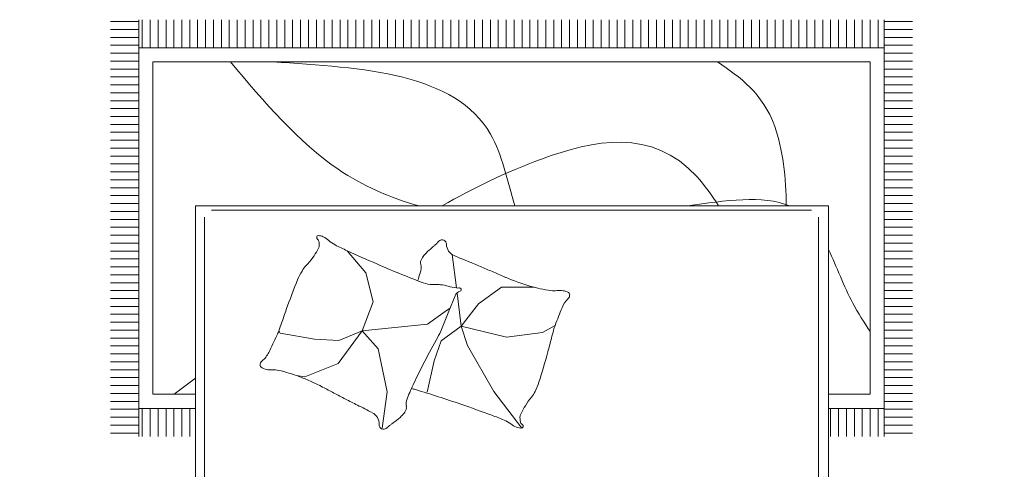
# Model space of a CAD drawing. Units: inches. Extents: x -7 to 1228, y -146 to 1091.
# Tile 78 of 88: x 656 to 743, y 890 to 929. Entities that reach past the tile are written whole.
import ezdxf

# ---------------------------------------------------------------- set-up
doc = ezdxf.new("R2010")
doc.units = ezdxf.units.IN
doc.layers.add('A-FURN', color=8, linetype='Continuous', lineweight=18)
doc.styles.add('DIM_FONT', font='SIMPLEX.shx', dxfattribs={"width": 0.8})

# ---------------------------------------------------------------- blocks, each defined once
blk = doc.blocks.new('A$C4F634EDD')
for p, q in [((0, 2.6295), (0, 2.2295)), ((0.5, 2.6295), (0, 2.6295)), ((0.5, 2.6295), (2.3, 2.6295)), ((0.5, 0.5295), (0.5, 2.6295)), ((0.5, 2.2295), (0.5, 2.6295)), ((2.3, 2.6295), (2.3, 0.5295)), ((2.3, 2.6295), (2.8, 2.6295)), ((2.3, 2.2295), (2.3, 2.6295)), ((2.8, 2.6295), (2.8, 2.2295)), ((0.5, 2.5771), (2.3, 2.5771)), ((2.392, 2.5115), (2.5692, 2.5765)), ((2.5692, 2.5765), (2.574, 2.5743)), ((0.2457, 2.5697), (0.2457, 2.4733)), ((2.4985, 2.5445), (2.5516, 2.564)), ((2.5062, 2.5454), (2.5487, 2.561)), ((2.5483, 2.5347), (2.5487, 2.561)), ((2.5487, 2.561), (2.5571, 2.56)), ((2.5615, 2.5536), (2.5514, 2.5318)), ((2.5516, 2.564), (2.5637, 2.5584)), ((2.5571, 2.56), (2.5615, 2.5536)), ((2.5615, 2.5536), (2.5791, 2.5058)), ((2.5637, 2.5584), (2.6418, 2.3458)), ((2.574, 2.5743), (2.6638, 2.3298)), ((2.4842, 2.5232), (2.47, 2.518)), ((2.4862, 2.5179), (2.4842, 2.5232)), ((2.4946, 2.5331), (2.4985, 2.5445)), ((2.5734, 2.3187), (2.4946, 2.5331)), ((2.5062, 2.5454), (2.5004, 2.5392)), ((2.5004, 2.5392), (2.5013, 2.5315)), ((2.5013, 2.5315), (2.5188, 2.4836)), ((2.5013, 2.5315), (2.5231, 2.5214)), ((2.5235, 2.5256), (2.5062, 2.5454)), ((2.5231, 2.5214), (2.5235, 2.5256)), ((2.5523, 2.4417), (2.5231, 2.5214)), ((2.5483, 2.5347), (2.5235, 2.5256)), ((2.5514, 2.5318), (2.5483, 2.5347)), ((2.5807, 2.4521), (2.5514, 2.5318)), ((2.3898, 2.5066), (2.392, 2.5115)), ((2.4795, 2.2621), (2.3898, 2.5066)), ((2.412, 2.5007), (2.4634, 2.5196)), ((2.4361, 2.4352), (2.412, 2.5007)), ((2.4634, 2.5196), (2.4875, 2.454)), ((2.47, 2.518), (2.472, 2.5127)), ((2.472, 2.5127), (2.4862, 2.5179)), ((2.4881, 2.5126), (2.4739, 2.5074)), ((2.4739, 2.5074), (2.4759, 2.502)), ((2.4759, 2.502), (2.4901, 2.5073)), ((2.492, 2.5019), (2.4778, 2.4967)), ((2.4778, 2.4967), (2.4798, 2.4914)), ((2.4798, 2.4914), (2.494, 2.4966)), ((2.4901, 2.5073), (2.4881, 2.5126)), ((2.494, 2.4966), (2.492, 2.5019)), ((2.5788, 2.4956), (2.5767, 2.4848)), ((2.5791, 2.5058), (2.5788, 2.4956)), ((2.4959, 2.4913), (2.4817, 2.4861)), ((2.4817, 2.4861), (2.4837, 2.4808)), ((2.4837, 2.4808), (2.4979, 2.486)), ((2.4998, 2.4807), (2.4856, 2.4755)), ((2.4856, 2.4755), (2.4876, 2.4702)), ((2.4876, 2.4702), (2.5018, 2.4754)), ((2.5037, 2.47), (2.4895, 2.4648)), ((2.4895, 2.4648), (2.4915, 2.4595)), ((2.4915, 2.4595), (2.5057, 2.4647)), ((2.4979, 2.486), (2.4959, 2.4913)), ((2.5018, 2.4754), (2.4998, 2.4807)), ((2.5057, 2.4647), (2.5037, 2.47)), ((2.5188, 2.4836), (2.5256, 2.4761)), ((2.5256, 2.4761), (2.5342, 2.4692)), ((2.5342, 2.4692), (2.5405, 2.4574)), ((2.5767, 2.4848), (2.5795, 2.4717)), ((2.5795, 2.4717), (2.586, 2.454)), ((2.4875, 2.454), (2.4361, 2.4352)), ((2.5405, 2.4574), (2.547, 2.4397)), ((2.5594, 2.4061), (2.547, 2.4397)), ((2.5523, 2.4417), (2.5875, 2.346)), ((2.5807, 2.4521), (2.6158, 2.3564)), ((2.5984, 2.4204), (2.586, 2.454)), ((0.0957, 2.4197), (0.192, 2.4197)), ((0.2994, 2.4197), (0.3957, 2.4197)), ((2.4457, 2.4146), (2.4563, 2.4185)), ((2.4496, 2.4039), (2.4457, 2.4146)), ((2.4563, 2.4185), (2.4602, 2.4078)), ((2.4634, 2.4211), (2.474, 2.425)), ((2.4673, 2.4104), (2.4634, 2.4211)), ((2.4779, 2.4143), (2.4673, 2.4104)), ((2.474, 2.425), (2.4779, 2.4143)), ((2.4811, 2.4276), (2.4917, 2.4315)), ((2.485, 2.4169), (2.4811, 2.4276)), ((2.4956, 2.4208), (2.485, 2.4169)), ((2.4883, 2.4081), (2.4989, 2.412)), ((2.4922, 2.3975), (2.4883, 2.4081)), ((2.4917, 2.4315), (2.4956, 2.4208)), ((2.4989, 2.412), (2.5028, 2.4014)), ((2.6047, 2.4086), (2.5984, 2.4204)), ((2.6133, 2.4017), (2.6047, 2.4086)), ((2.4602, 2.4078), (2.4496, 2.4039)), ((2.4528, 2.3951), (2.4635, 2.399)), ((2.4567, 2.3844), (2.4528, 2.3951)), ((2.4674, 2.3883), (2.4567, 2.3844)), ((2.4635, 2.399), (2.4674, 2.3883)), ((2.4706, 2.4016), (2.4812, 2.4055)), ((2.4745, 2.3909), (2.4706, 2.4016)), ((2.4851, 2.3949), (2.4745, 2.3909)), ((2.4777, 2.3821), (2.4883, 2.386)), ((2.4816, 2.3715), (2.4777, 2.3821)), ((2.4812, 2.4055), (2.4851, 2.3949)), ((2.4883, 2.386), (2.4922, 2.3754)), ((2.5028, 2.4014), (2.4922, 2.3975)), ((2.4954, 2.3886), (2.5061, 2.3925)), ((2.4993, 2.378), (2.4954, 2.3886)), ((2.51, 2.3819), (2.4993, 2.378)), ((2.5061, 2.3925), (2.51, 2.3819)), ((2.5238, 2.3769), (2.538, 2.3821)), ((2.538, 2.3821), (2.5419, 2.3715)), ((2.5622, 2.393), (2.5594, 2.4061)), ((2.5598, 2.372), (2.5601, 2.3822)), ((2.5601, 2.3822), (2.5622, 2.393)), ((2.6201, 2.3941), (2.6133, 2.4017)), ((2.6376, 2.3463), (2.6201, 2.3941)), ((2.6499, 2.3979), (2.6397, 2.3953)), ((2.6417, 2.39), (2.6488, 2.391)), ((2.6488, 2.391), (2.6538, 2.3895)), ((2.6551, 2.397), (2.6499, 2.3979)), ((2.6538, 2.3895), (2.6596, 2.388)), ((2.6627, 2.392), (2.6551, 2.397)), ((2.6596, 2.388), (2.6626, 2.3867)), ((2.6626, 2.3867), (2.6662, 2.388)), ((2.6692, 2.394), (2.6627, 2.392)), ((2.6662, 2.388), (2.6632, 2.3828)), ((2.6632, 2.3828), (2.6736, 2.3744)), ((2.6736, 2.3944), (2.6692, 2.394)), ((2.6765, 2.391), (2.6736, 2.3944)), ((2.6742, 2.3795), (2.6765, 2.391)), ((2.6824, 2.3858), (2.6742, 2.3795)), ((2.6873, 2.3815), (2.6824, 2.3858)), ((2.6853, 2.369), (2.6873, 2.3815)), ((0.2457, 2.366), (0.2457, 2.2697)), ((2.46, 2.3756), (2.4706, 2.3795)), ((2.4639, 2.365), (2.46, 2.3756)), ((2.4745, 2.3689), (2.4639, 2.365)), ((2.4672, 2.3561), (2.4778, 2.36)), ((2.4711, 2.3455), (2.4672, 2.3561)), ((2.4706, 2.3795), (2.4745, 2.3689)), ((2.4778, 2.36), (2.4817, 2.3494)), ((2.4922, 2.3754), (2.4816, 2.3715)), ((2.4849, 2.3626), (2.4955, 2.3665)), ((2.4888, 2.352), (2.4849, 2.3626)), ((2.4994, 2.3559), (2.4888, 2.352)), ((2.4955, 2.3665), (2.4994, 2.3559)), ((2.5026, 2.3691), (2.5132, 2.373)), ((2.5065, 2.3585), (2.5026, 2.3691)), ((2.5171, 2.3624), (2.5065, 2.3585)), ((2.5132, 2.373), (2.5171, 2.3624)), ((2.5277, 2.3663), (2.5238, 2.3769)), ((2.5419, 2.3715), (2.5277, 2.3663)), ((2.5774, 2.3242), (2.5598, 2.372)), ((2.6154, 2.3522), (2.5905, 2.3431)), ((2.6158, 2.3564), (2.6154, 2.3522)), ((2.6154, 2.3522), (2.6327, 2.3324)), ((2.6376, 2.3463), (2.6158, 2.3564)), ((2.6736, 2.3744), (2.6922, 2.3593)), ((2.6946, 2.376), (2.6853, 2.369)), ((2.6922, 2.3593), (2.7051, 2.3473)), ((2.6995, 2.3713), (2.6946, 2.376)), ((2.695, 2.3603), (2.6995, 2.3713)), ((2.7031, 2.3682), (2.695, 2.3603)), ((2.7096, 2.3616), (2.7031, 2.3682)), ((2.7062, 2.351), (2.7096, 2.3616)), ((2.7147, 2.3578), (2.7062, 2.351)), ((2.7214, 2.3517), (2.7147, 2.3578)), ((0, 2.3301), (0.5, 2.3301)), ((2.8, 2.3301), (2.3, 2.3301)), ((2.4817, 2.3494), (2.4711, 2.3455)), ((2.5774, 2.3242), (2.5875, 2.346)), ((2.5818, 2.3178), (2.5774, 2.3242)), ((2.5875, 2.346), (2.5905, 2.3431)), ((2.5905, 2.3431), (2.5901, 2.3168)), ((2.5901, 2.3168), (2.6097, 2.324)), ((2.613, 2.3312), (2.6077, 2.3293)), ((2.6077, 2.3293), (2.6135, 2.3141)), ((2.6192, 2.3174), (2.613, 2.3312)), ((2.6153, 2.3261), (2.6327, 2.3324)), ((2.6369, 2.332), (2.6161, 2.3243)), ((2.6616, 2.3249), (2.6234, 2.3109)), ((2.6327, 2.3324), (2.6385, 2.3386)), ((2.6418, 2.3458), (2.6369, 2.332)), ((2.6385, 2.3386), (2.6376, 2.3463)), ((2.6638, 2.3298), (2.6616, 2.3249)), ((2.7051, 2.3473), (2.7079, 2.3475)), ((2.7079, 2.3475), (2.7079, 2.3443)), ((2.7079, 2.3443), (2.727, 2.3277)), ((2.7196, 2.34), (2.7214, 2.3517)), ((2.7286, 2.3466), (2.7196, 2.34)), ((2.727, 2.3277), (2.7512, 2.2983)), ((2.7346, 2.3423), (2.7286, 2.3466)), ((2.732, 2.3295), (2.7346, 2.3423)), ((2.7423, 2.3345), (2.732, 2.3295)), ((2.7406, 2.3172), (2.7495, 2.325)), ((2.7495, 2.325), (2.7423, 2.3345)), ((2.6172, 2.3086), (2.4844, 2.2599)), ((2.5362, 2.305), (2.5185, 2.2985)), ((2.5185, 2.2985), (2.5224, 2.2879)), ((2.5401, 2.2944), (2.5362, 2.305)), ((2.561, 2.3141), (2.5433, 2.3076)), ((2.5433, 2.3076), (2.5472, 2.297)), ((2.5472, 2.297), (2.5649, 2.3035)), ((2.5649, 2.3035), (2.561, 2.3141)), ((2.5855, 2.3131), (2.5734, 2.3187)), ((2.5901, 2.3168), (2.5818, 2.3178)), ((2.6104, 2.3222), (2.5855, 2.3131)), ((2.6135, 2.3141), (2.6244, 2.2977)), ((2.626, 2.3069), (2.6192, 2.3174)), ((2.6244, 2.2977), (2.6349, 2.2825)), ((2.6365, 2.2916), (2.626, 2.3069)), ((2.7519, 2.3218), (2.7406, 2.3172)), ((2.7512, 2.2983), (2.756, 2.2695)), ((2.7575, 2.3144), (2.7519, 2.3218)), ((2.7526, 2.3045), (2.7575, 2.3144)), ((2.7622, 2.308), (2.7526, 2.3045)), ((2.7574, 2.2924), (2.7673, 2.2997)), ((2.7673, 2.2997), (2.7622, 2.308)), ((0.5953, 2.1912), (0.616, 2.2738)), ((1.4546, 2.1912), (1.4752, 2.2738)), ((2.5114, 2.2959), (2.4936, 2.2894)), ((2.4936, 2.2894), (2.4976, 2.2788)), ((2.4976, 2.2788), (2.5153, 2.2853)), ((2.5153, 2.2853), (2.5114, 2.2959)), ((2.5224, 2.2879), (2.5401, 2.2944)), ((2.6349, 2.2825), (2.638, 2.273)), ((2.6407, 2.2834), (2.6365, 2.2916)), ((2.6399, 2.2712), (2.6374, 2.2659)), ((2.638, 2.273), (2.6399, 2.2712)), ((2.6438, 2.2739), (2.6407, 2.2834)), ((2.6519, 2.2716), (2.6438, 2.2739)), ((2.6535, 2.2628), (2.6519, 2.2716)), ((2.756, 2.2695), (2.7459, 2.2483)), ((2.7687, 2.2905), (2.7574, 2.2924)), ((2.7587, 2.279), (2.7699, 2.2828)), ((2.7708, 2.2725), (2.7587, 2.279)), ((2.7699, 2.2828), (2.7687, 2.2905)), ((2.7706, 2.2643), (2.7708, 2.2725)), ((2.4844, 2.2599), (2.4795, 2.2621)), ((2.6374, 2.2659), (2.6398, 2.257)), ((2.6398, 2.257), (2.6509, 2.259)), ((2.6509, 2.259), (2.6431, 2.2492)), ((2.6431, 2.2492), (2.6473, 2.2398)), ((2.6473, 2.2398), (2.6592, 2.2429)), ((2.6592, 2.2429), (2.6521, 2.2314)), ((2.6636, 2.2409), (2.6535, 2.2628)), ((2.6836, 2.2287), (2.6636, 2.2409)), ((2.7459, 2.2483), (2.7284, 2.2317)), ((2.7509, 2.2314), (2.7459, 2.2418)), ((2.7459, 2.2418), (2.7568, 2.2352)), ((2.7529, 2.2505), (2.7645, 2.2498)), ((2.7607, 2.2424), (2.7529, 2.2505)), ((2.7568, 2.2352), (2.7607, 2.2424)), ((2.759, 2.2637), (2.7706, 2.2643)), ((2.7676, 2.2559), (2.759, 2.2637)), ((2.7645, 2.2498), (2.7676, 2.2559)), ((0, 2.2295), (0.5, 2.2295)), ((2.8, 2.2295), (2.3, 2.2295)), ((2.6521, 2.2314), (2.6598, 2.2248)), ((2.6598, 2.2248), (2.6697, 2.2309)), ((2.6697, 2.2309), (2.6684, 2.219)), ((2.6684, 2.219), (2.6761, 2.2145)), ((2.6761, 2.2145), (2.6821, 2.2237)), ((2.6821, 2.2237), (2.6843, 2.2135)), ((2.7063, 2.2256), (2.6836, 2.2287)), ((2.6843, 2.2135), (2.6927, 2.2117)), ((2.6927, 2.2117), (2.6986, 2.222)), ((2.6986, 2.222), (2.7019, 2.2098)), ((2.7284, 2.2317), (2.7063, 2.2256)), ((2.7102, 2.2104), (2.7113, 2.2218)), ((2.7113, 2.2218), (2.7192, 2.2137)), ((2.7192, 2.2137), (2.7255, 2.2152)), ((2.7255, 2.2152), (2.7242, 2.2265)), ((2.7242, 2.2265), (2.7324, 2.2165)), ((2.7324, 2.2165), (2.7386, 2.2208)), ((2.7386, 2.2208), (2.7354, 2.2306)), ((2.7354, 2.2306), (2.7462, 2.2264)), ((2.7462, 2.2264), (2.7509, 2.2314)), ((0.5878, 2.1612), (0.5953, 2.1912)), ((1.4471, 2.1612), (1.4546, 2.1912)), ((2.7019, 2.2098), (2.7102, 2.2104)), ((1.5035, 2.141), (0.5458, 2.141)), ((1.5035, 2.141), (2.2716, 1.7136)), ((0.5258, 2.121), (0.5258, 0.5617)), ((1.576, 1.9433), (1.5624, 1.8479)), ((0.5458, 1.8684), (1.5653, 1.8684)), ((1.5624, 1.8479), (1.5641, 1.7178)), ((2.2716, 0.5617), (2.2716, 1.7136)), ((0.3386, 0), (0.3386, 1.1852)), ((0.3486, 1.1052), (0.3486, 1.1852)), ((0.3711, 1.1052), (0.3711, 1.1852)), ((0.3936, 1.1052), (0.3936, 1.1852)), ((0.4161, 1.1052), (0.4161, 1.1852)), ((0.4386, 1.1052), (0.4386, 1.1852)), ((0.4611, 1.1052), (0.4611, 1.1852)), ((0.4836, 1.1052), (0.4836, 1.1852)), ((2.3061, 1.1052), (2.3061, 1.1852)), ((2.3286, 1.1052), (2.3286, 1.1852)), ((2.3511, 1.1052), (2.3511, 1.1852)), ((2.3736, 1.1052), (2.3736, 1.1852)), ((2.3961, 1.1052), (2.3961, 1.1852)), ((2.4186, 1.1052), (2.4186, 1.1852)), ((2.4411, 1.1052), (2.4411, 1.1852)), ((2.4588, 1.1852), (2.4588, 0)), ((0.2586, 1.1753), (0.3386, 1.1753)), ((0.2586, 1.1528), (0.3386, 1.1528)), ((1.031, 1.1612), (1.0448, 1.0581)), ((1.4276, 1.1611), (1.3484, 1.0571)), ((2.4588, 1.1753), (2.5388, 1.1753)), ((2.4588, 1.1528), (2.5388, 1.1528)), ((0.2586, 1.1303), (0.3386, 1.1303)), ((2.4588, 1.1303), (2.5388, 1.1303)), ((0.2586, 1.1078), (0.3386, 1.1078)), ((0.3386, 1.1052), (0.5, 1.1052)), ((2.3, 1.1052), (2.4588, 1.1052)), ((2.4588, 1.1078), (2.5388, 1.1078)), ((0.2586, 1.0853), (0.3386, 1.0853)), ((0.3786, 1.0652), (0.5, 1.0652)), ((0.3786, 0.12), (0.3786, 1.0652)), ((2.3, 1.0652), (2.4188, 1.0652)), ((2.4188, 1.0652), (2.4188, 0.12)), ((2.4588, 1.0853), (2.5388, 1.0853)), ((0.2586, 1.0628), (0.3386, 1.0628)), ((0.2586, 1.0403), (0.3386, 1.0403)), ((1.0448, 1.0581), (1.019, 0.936)), ((1.1784, 0.9702), (1.1586, 1.0591)), ((1.3484, 1.0571), (1.2733, 0.9268)), ((2.4588, 1.0628), (2.5388, 1.0628)), ((2.4588, 1.0403), (2.5388, 1.0403)), ((0.2586, 1.0178), (0.3386, 1.0178)), ((0.8108, 1.0151), (0.7868, 1.0117)), ((0.9054, 0.9773), (0.8108, 1.0151)), ((2.4588, 1.0178), (2.5388, 1.0178)), ((0.2586, 0.9953), (0.3386, 0.9953)), ((2.4588, 0.9953), (2.5388, 0.9953)), ((0.2586, 0.9728), (0.3386, 0.9728)), ((0.9743, 0.8845), (0.9054, 0.9773)), ((1.1982, 0.9129), (1.1784, 0.9702)), ((2.4588, 0.9728), (2.5388, 0.9728)), ((0.2586, 0.9503), (0.3386, 0.9503)), ((0.2586, 0.9278), (0.3386, 0.9278)), ((1.019, 0.936), (0.9743, 0.8845)), ((1.2733, 0.9268), (1.2555, 0.8715)), ((2.4588, 0.9503), (2.5388, 0.9503)), ((2.4588, 0.9278), (2.5388, 0.9278)), ((0.2586, 0.9053), (0.3386, 0.9053)), ((0.8384, 0.9085), (0.7403, 0.8913)), ((0.9072, 0.912), (0.8384, 0.9085)), ((0.9743, 0.8845), (0.9072, 0.912)), ((1.2555, 0.8715), (1.1982, 0.9129)), ((1.2555, 0.8715), (1.384, 0.9031)), ((1.384, 0.9031), (1.4868, 0.8892)), ((2.4588, 0.9053), (2.5388, 0.9053)), ((0.2586, 0.8828), (0.3386, 0.8828)), ((0.7403, 0.8913), (0.737, 0.8849)), ((0.9743, 0.8845), (1.0052, 0.802)), ((0.9743, 0.8845), (1.16, 0.8656)), ((1.1973, 0.8853), (1.2203, 0.829)), ((1.2555, 0.8715), (1.2437, 0.7773)), ((1.2555, 0.8715), (1.3049, 0.8082)), ((1.4868, 0.8892), (1.5228, 0.8692)), ((2.4588, 0.8828), (2.5388, 0.8828)), ((0.2586, 0.8603), (0.3386, 0.8603)), ((1.16, 0.8656), (1.2099, 0.8295)), ((2.4588, 0.8603), (2.5388, 0.8603)), ((0.2586, 0.8378), (0.3386, 0.8378)), ((0.2586, 0.8153), (0.3386, 0.8153)), ((1.2099, 0.8295), (1.222, 0.8209)), ((1.2203, 0.829), (1.2381, 0.7855)), ((2.4588, 0.8378), (2.5388, 0.8378)), ((2.4588, 0.8153), (2.5388, 0.8153)), ((0.2586, 0.7928), (0.3386, 0.7928)), ((1.0052, 0.802), (0.9846, 0.7194)), ((1.3049, 0.8082), (1.3701, 0.7608)), ((2.4588, 0.7928), (2.5388, 0.7928)), ((0.2586, 0.7703), (0.3386, 0.7703)), ((1.2419, 0.7626), (1.23, 0.668)), ((1.3701, 0.7608), (1.463, 0.7608)), ((2.4588, 0.7703), (2.5388, 0.7703)), ((0.2586, 0.7478), (0.3386, 0.7478)), ((2.4588, 0.7478), (2.5388, 0.7478)), ((0.2586, 0.7253), (0.3386, 0.7253)), ((0.2586, 0.7028), (0.3386, 0.7028)), ((0.9846, 0.7194), (0.931, 0.6569)), ((2.4588, 0.7253), (2.5388, 0.7253)), ((2.4588, 0.7028), (2.5388, 0.7028)), ((0.2586, 0.6803), (0.3386, 0.6803)), ((2.4588, 0.6803), (2.5388, 0.6803)), ((0.2586, 0.6578), (0.3386, 0.6578)), ((2.4588, 0.6578), (2.5388, 0.6578)), ((0.2586, 0.6353), (0.3386, 0.6353)), ((2.4588, 0.6353), (2.5388, 0.6353)), ((0.2586, 0.6128), (0.3386, 0.6128)), ((0.2586, 0.5903), (0.3386, 0.5903)), ((2.4588, 0.6128), (2.5388, 0.6128)), ((2.4588, 0.5903), (2.5388, 0.5903)), ((0.2586, 0.5678), (0.3386, 0.5678)), ((2.4588, 0.5678), (2.5388, 0.5678)), ((0.2586, 0.5453), (0.3386, 0.5453)), ((0.5458, 0.5417), (2.2516, 0.5417)), ((2.4588, 0.5453), (2.5388, 0.5453)), ((0.2586, 0.5228), (0.3386, 0.5228)), ((2.3, 0.5295), (0.5, 0.5295)), ((2.4588, 0.5228), (2.5388, 0.5228)), ((0.2586, 0.5003), (0.3386, 0.5003)), ((0.2586, 0.4778), (0.3386, 0.4778)), ((2.4588, 0.5003), (2.5388, 0.5003)), ((2.4588, 0.4778), (2.5388, 0.4778)), ((0.2586, 0.4553), (0.3386, 0.4553)), ((2.4588, 0.4553), (2.5388, 0.4553)), ((0.2586, 0.4328), (0.3386, 0.4328)), ((2.4588, 0.4328), (2.5388, 0.4328)), ((0.2586, 0.4103), (0.3386, 0.4103)), ((2.4588, 0.4103), (2.5388, 0.4103)), ((0.2586, 0.3878), (0.3386, 0.3878)), ((0.2586, 0.3653), (0.3386, 0.3653)), ((2.4588, 0.3878), (2.5388, 0.3878)), ((2.4588, 0.3653), (2.5388, 0.3653)), ((0.2586, 0.3428), (0.3386, 0.3428)), ((2.4588, 0.3428), (2.5388, 0.3428)), ((0.2586, 0.3203), (0.3386, 0.3203)), ((2.4588, 0.3203), (2.5388, 0.3203)), ((0.2586, 0.2978), (0.3386, 0.2978)), ((2.4588, 0.2978), (2.5388, 0.2978)), ((0.2586, 0.2753), (0.3386, 0.2753)), ((0.2586, 0.2528), (0.3386, 0.2528)), ((2.4588, 0.2753), (2.5388, 0.2753)), ((2.4588, 0.2528), (2.5388, 0.2528)), ((0.2586, 0.2303), (0.3386, 0.2303)), ((2.4588, 0.2303), (2.5388, 0.2303)), ((0.2586, 0.2078), (0.3386, 0.2078)), ((2.4588, 0.2078), (2.5388, 0.2078)), ((0.2586, 0.1853), (0.3386, 0.1853)), ((2.4588, 0.1853), (2.5388, 0.1853)), ((0.2586, 0.1628), (0.3386, 0.1628)), ((0.2586, 0.1403), (0.3386, 0.1403)), ((2.4588, 0.1628), (2.5388, 0.1628)), ((2.4588, 0.1403), (2.5388, 0.1403)), ((0.2586, 0.1178), (0.3386, 0.1178)), ((2.4188, 0.12), (0.3786, 0.12)), ((2.4588, 0.1178), (2.5388, 0.1178)), ((0.2586, 0.0953), (0.3386, 0.0953)), ((2.4588, 0.0953), (2.5388, 0.0953)), ((0.2586, 0.0728), (0.3386, 0.0728)), ((2.4588, 0.08), (0.3386, 0.08)), ((0.3486, 0), (0.3486, 0.08)), ((0.3711, 0), (0.3711, 0.08)), ((0.3936, 0), (0.3936, 0.08)), ((0.4161, 0), (0.4161, 0.08)), ((0.4386, 0), (0.4386, 0.08)), ((0.4611, 0), (0.4611, 0.08)), ((0.4836, 0), (0.4836, 0.08)), ((0.5061, 0), (0.5061, 0.08)), ((0.5286, 0), (0.5286, 0.08)), ((0.5511, 0), (0.5511, 0.08)), ((0.5736, 0), (0.5736, 0.08)), ((0.5961, 0), (0.5961, 0.08)), ((0.6186, 0), (0.6186, 0.08)), ((0.6411, 0), (0.6411, 0.08)), ((0.6636, 0), (0.6636, 0.08)), ((0.6861, 0), (0.6861, 0.08)), ((0.7086, 0), (0.7086, 0.08)), ((0.7311, 0), (0.7311, 0.08)), ((0.7536, 0), (0.7536, 0.08)), ((0.7761, 0), (0.7761, 0.08)), ((0.7986, 0), (0.7986, 0.08)), ((0.8211, 0), (0.8211, 0.08)), ((0.8436, 0), (0.8436, 0.08)), ((0.8661, 0), (0.8661, 0.08)), ((0.8886, 0), (0.8886, 0.08)), ((0.9111, 0), (0.9111, 0.08)), ((0.9336, 0), (0.9336, 0.08)), ((0.9561, 0), (0.9561, 0.08)), ((0.9786, 0), (0.9786, 0.08)), ((1.0011, 0), (1.0011, 0.08)), ((1.0236, 0), (1.0236, 0.08)), ((1.0461, 0), (1.0461, 0.08)), ((1.0686, 0), (1.0686, 0.08)), ((1.0911, 0), (1.0911, 0.08)), ((1.1136, 0), (1.1136, 0.08)), ((1.1361, 0), (1.1361, 0.08)), ((1.1586, 0), (1.1586, 0.08)), ((1.1811, 0), (1.1811, 0.08)), ((1.2036, 0), (1.2036, 0.08)), ((1.2261, 0), (1.2261, 0.08)), ((1.2486, 0), (1.2486, 0.08)), ((1.2711, 0), (1.2711, 0.08)), ((1.2936, 0), (1.2936, 0.08)), ((1.3161, 0), (1.3161, 0.08)), ((1.3386, 0), (1.3386, 0.08)), ((1.3611, 0), (1.3611, 0.08)), ((1.3836, 0), (1.3836, 0.08)), ((1.4061, 0), (1.4061, 0.08)), ((1.4286, 0), (1.4286, 0.08)), ((1.4511, 0), (1.4511, 0.08)), ((1.4736, 0), (1.4736, 0.08)), ((1.4961, 0), (1.4961, 0.08)), ((1.5186, 0), (1.5186, 0.08)), ((1.5411, 0), (1.5411, 0.08)), ((1.5636, 0), (1.5636, 0.08)), ((1.5861, 0), (1.5861, 0.08)), ((1.6086, 0), (1.6086, 0.08)), ((1.6311, 0), (1.6311, 0.08)), ((1.6536, 0), (1.6536, 0.08)), ((1.6761, 0), (1.6761, 0.08)), ((1.6986, 0), (1.6986, 0.08)), ((1.7211, 0), (1.7211, 0.08)), ((1.7436, 0), (1.7436, 0.08)), ((1.7661, 0), (1.7661, 0.08)), ((1.7886, 0), (1.7886, 0.08)), ((1.8111, 0), (1.8111, 0.08)), ((1.8336, 0), (1.8336, 0.08)), ((1.8561, 0), (1.8561, 0.08)), ((1.8786, 0), (1.8786, 0.08)), ((1.9011, 0), (1.9011, 0.08)), ((1.9236, 0), (1.9236, 0.08)), ((1.9461, 0), (1.9461, 0.08)), ((1.9686, 0), (1.9686, 0.08)), ((1.9911, 0), (1.9911, 0.08)), ((2.0136, 0), (2.0136, 0.08)), ((2.0361, 0), (2.0361, 0.08)), ((2.0586, 0), (2.0586, 0.08)), ((2.0811, 0), (2.0811, 0.08)), ((2.1036, 0), (2.1036, 0.08)), ((2.1261, 0), (2.1261, 0.08)), ((2.1486, 0), (2.1486, 0.08)), ((2.1711, 0), (2.1711, 0.08)), ((2.1936, 0), (2.1936, 0.08)), ((2.2161, 0), (2.2161, 0.08)), ((2.2386, 0), (2.2386, 0.08)), ((2.2611, 0), (2.2611, 0.08)), ((2.2836, 0), (2.2836, 0.08)), ((2.3061, 0), (2.3061, 0.08)), ((2.3286, 0), (2.3286, 0.08)), ((2.3511, 0), (2.3511, 0.08)), ((2.3736, 0), (2.3736, 0.08)), ((2.3961, 0), (2.3961, 0.08)), ((2.4186, 0), (2.4186, 0.08)), ((2.4411, 0), (2.4411, 0.08)), ((2.4588, 0.0728), (2.5388, 0.0728)), ((0.2586, 0.0503), (0.3386, 0.0503)), ((2.4588, 0.0503), (2.5388, 0.0503)), ((0.2586, 0.0278), (0.3386, 0.0278)), ((0.2586, 0.0053), (0.3386, 0.0053)), ((2.4588, 0.0278), (2.5388, 0.0278)), ((2.4588, 0.0053), (2.5388, 0.0053))]:
    blk.add_line(p, q)
for radius in [0.1222, 0.0865]:
    blk.add_circle((0.2457, 2.4197), radius)
for centre, radius, start, end in [((0.5848, 2.5274), 0.0131, 101.2724, 206.5805), ((0.6036, 2.5368), 0.0342, 206.5805, 265.5998), ((0.5999, 2.4516), 0.0904, 90, 101.2724), ((0.5999, 2.3808), 0.1611, 81.5628, 90), ((0.5788, 2.2388), 0.3048, 74.256, 81.5628), ((0.7272, 2.7653), 0.2422, 254.256, 262.4531), ((0.7851, 3.2019), 0.6827, 262.4531, 270), ((0.7851, 3.5682), 1.049, 270, 276.0867), ((0.8402, 3.0514), 0.5293, 276.0867, 280.1899), ((1.1602, -8.1346), 10.6675, 90.30153, 91.21582), ((1.1169, 2.2433), 0.2897, 85.1982, 92.5386), ((1.2142, 3.4021), 0.8732, 265.1982, 269.4243), ((1.3082, 2.3102), 0.234, 110.8603, 117.2396), ((1.2204, 4.0232), 1.4943, 269.4243, 271.9079), ((1.2995, 2.4357), 0.0992, 105.9352, 126.0864), ((1.2429, 3.3501), 0.8208, 271.9079, 275.2592), ((1.2995, 2.4357), 0.0992, 85.7841, 105.9352), ((1.3132, 2.5864), 0.0539, 275.2592, 300.6513), ((1.3554, 2.5152), 0.0289, 85.6975, 120.6513), ((1.3556, 2.519), 0.0251, 68.2117, 85.6975), ((1.3739, 2.5288), 0.0156, 158.0096, 201.421), ((1.3634, 2.533), 0.00428, 78.1069, 158.0096), ((1.3288, 2.5111), 0.0328, 351.8665, 21.421), ((1.3647, 2.5395), 0.00232, 258.1069, 19.564), ((1.3637, 2.5391), 0.00342, 19.564, 68.2117), ((1.444, 2.5274), 0.0131, 101.2724, 206.5805), ((1.4628, 2.5368), 0.0342, 206.5805, 265.5998), ((1.4591, 2.4516), 0.0904, 90, 101.2724), ((1.4591, 2.3808), 0.1611, 81.5628, 90), ((1.438, 2.2388), 0.3048, 74.256, 81.5628), ((1.5865, 2.7653), 0.2422, 254.256, 262.4531), ((1.6443, 3.2019), 0.6827, 262.4531, 270), ((1.6443, 3.5682), 1.049, 270, 276.0867), ((1.4785, 15.4878), 12.9656, 271.22425, 272.05324), ((1.97, 2.3805), 0.1524, 92.5386, 100.1899), ((1.9761, 2.2433), 0.2897, 85.1982, 92.5386), ((2.0734, 3.4021), 0.8732, 265.1982, 269.4243), ((2.1674, 2.3102), 0.234, 110.8603, 117.2396), ((2.0797, 4.0232), 1.4943, 269.4243, 271.9079), ((2.1588, 2.4357), 0.0992, 105.9352, 126.0864), ((2.1021, 3.3501), 0.8208, 271.9079, 275.2592), ((2.1588, 2.4357), 0.0992, 85.7841, 105.9352), ((2.1724, 2.5864), 0.0539, 275.2592, 300.6513), ((2.2146, 2.5152), 0.0289, 85.6975, 120.6513), ((2.2149, 2.519), 0.0251, 68.2117, 85.6975), ((2.2331, 2.5288), 0.0156, 158.0096, 201.421), ((2.2226, 2.533), 0.00428, 78.1069, 158.0096), ((2.1881, 2.5111), 0.0328, 351.8665, 21.421), ((2.224, 2.5395), 0.00232, 258.1069, 19.564), ((2.2229, 2.5391), 0.00342, 19.564, 68.2117), ((1.0898, 2.4496), 0.4918, 173.7676, 180), ((0.5368, 2.3783), 0.1399, 45.0976, 62.7964), ((1.4317, 2.2032), 0.3916, 128.3886, 133.8115), ((1.2362, 2.45), 0.0768, 117.2396, 128.3886), ((1.2995, 2.4357), 0.0992, 143.8234, 161.5603), ((1.2995, 2.4357), 0.0992, 126.0864, 143.8234), ((1.1177, 2.5413), 0.246, 347.8905, 351.8665), ((1.949, 2.4496), 0.4918, 173.7676, 180), ((2.291, 2.2032), 0.3916, 128.3886, 133.8115), ((2.0954, 2.45), 0.0768, 117.2396, 128.3886), ((2.1588, 2.4357), 0.0992, 143.8234, 161.5603), ((2.1588, 2.4357), 0.0992, 126.0864, 143.8234), ((1.977, 2.5413), 0.246, 347.8905, 351.8665), ((0.5462, 2.4142), 0.0899, 41.4429, 53.7359), ((0.5741, 2.4389), 0.0526, 25.3551, 41.4429), ((0.5368, 2.3783), 0.1399, 27.3988, 45.0976), ((1.1799, 2.4341), 0.0493, 140.9651, 151.6832), ((1.3165, 2.3233), 0.2252, 133.8115, 140.9651), ((2.2605, 2.3525), 0.9131, 172.3191, 176.6313), ((1.5522, 2.448), 0.1983, 167.8905, 172.3191), ((2.0391, 2.4341), 0.0493, 140.9651, 151.6832), ((2.1757, 2.3233), 0.2252, 133.8115, 140.9651), ((3.1198, 2.3525), 0.9131, 172.3191, 176.6313), ((2.4114, 2.448), 0.1983, 167.8905, 172.3191), ((0.8019, 2.4496), 0.204, 180, 189.6844), ((0.4851, 2.3967), 0.1511, 21.8149, 25.3551), ((0.4345, 2.3765), 0.2056, 18.7799, 21.8149), ((0.576, 2.4246), 0.0562, 0, 18.7799), ((0.5368, 2.3783), 0.1399, 16.515, 27.3988), ((1.3127, 2.3625), 0.2002, 151.6832, 156.9972), ((1.6611, 2.4496), 0.204, 180, 189.6844), ((2.1719, 2.3625), 0.2002, 151.6832, 156.9972), ((1.4703, 2.5637), 0.882, 189.6844, 192.1984), ((0.5406, 2.4246), 0.0915, 345.3149, 0), ((0.5368, 2.3783), 0.1399, 5.6311, 16.515), ((2.3295, 2.5637), 0.882, 189.6844, 192.1984), ((2.0266, 2.3663), 0.6787, 176.6313, 181.6331), ((2.8858, 2.3663), 0.6787, 176.6313, 181.6331), ((0.2982, 2.3103), 0.3171, 8.0051, 12.1984), ((-0.0401, 2.2627), 0.6588, 2.6649, 8.0051), ((1.1575, 2.3103), 0.3171, 8.0051, 12.1984), ((0.8191, 2.2627), 0.6588, 2.6649, 8.0051), ((2.7128, 2.3859), 1.3652, 181.6331, 183.055), ((3.5721, 2.3859), 1.3652, 181.6331, 183.055), ((14.9657, 3.0398), 13.6356, 183.05496, 183.50486), ((15.8249, 3.0398), 13.6356, 183.05496, 183.50486), ((0.5503, 2.2902), 0.0677, 345.9548, 2.6649), ((1.4096, 2.2902), 0.0677, 345.9548, 2.6649), ((1.1303, 1.9835), 0.2721, 85.9172, 93.5552), ((1.1455, 2.197), 0.058, 69.3257, 85.9172), ((0.9871, 1.7772), 0.5066, 65.6735, 69.3257), ((0.473, 2.8815), 0.7387, 293.4844, 295.3111), ((0.6058, 0.9338), 1.4323, 63.5015, 65.6735), ((1.1054, 1.9358), 0.3126, 57.865, 63.5015), ((1.3322, 2.8815), 0.7387, 293.4844, 295.3111), ((0.473, 2.8815), 0.7387, 287.1982, 289.428), ((0.473, 2.8815), 0.7387, 289.428, 291.6577), ((0.473, 2.8815), 0.7387, 291.6577, 293.4844), ((0.8841, 1.5835), 0.7286, 54.1737, 57.865), ((1.6762, 2.2258), 0.3212, 183.5049, 189.9984), ((1.3322, 2.8815), 0.7387, 287.1982, 289.428), ((1.3322, 2.8815), 0.7387, 289.428, 291.6577), ((1.3322, 2.8815), 0.7387, 291.6577, 293.4844), ((2.5355, 2.2258), 0.3212, 183.5049, 189.9984), ((0.5887, 2.1609), 0.000917, 165.9551, 274.0829), ((0.5695, 2.4301), 0.2708, 274.0829, 279.4841), ((0.5763, 2.3896), 0.2297, 279.4841, 287.3864), ((0.6807, 2.0561), 0.1197, 96.4341, 107.3864), ((0.6836, 2.0301), 0.1459, 78.4414, 96.4341), ((0.759, 2.3985), 0.2301, 258.4414, 272.7491), ((0.7026, 3.5718), 1.4048, 272.7491, 274.6176), ((0.9136, 0.9591), 1.2165, 92.6096, 94.6176), ((1.2501, -19.8405), 22.0183, 90.37908, 91.01965), ((1.2012, -3.5404), 5.7185, 89.7135, 90.9704), ((1.224, 1.0141), 1.164, 86.426, 89.7135), ((1.2875, 2.0302), 0.1459, 77.131, 86.426), ((1.3099, 2.1283), 0.0453, 62.7159, 77.131), ((1.3658, 2.2367), 0.0767, 242.7159, 253.7788), ((1.3688, 2.247), 0.0875, 253.7788, 262.8796), ((1.3581, 2.1615), 0.00132, 262.8796, 343.3022), ((1.3409, 2.1667), 0.0193, 343.3022, 9.9984), ((1.448, 2.1609), 0.000917, 165.9551, 274.0829), ((1.4288, 2.4301), 0.2708, 274.0829, 279.4841), ((1.4355, 2.3896), 0.2297, 279.4841, 287.3864), ((1.5399, 2.0561), 0.1197, 96.4341, 107.3864), ((1.5429, 2.0301), 0.1459, 78.4414, 96.4341), ((1.6182, 2.3985), 0.2301, 258.4414, 272.7491), ((1.5619, 3.5718), 1.4048, 272.7491, 274.6176), ((1.7729, 0.9591), 1.2165, 92.6096, 94.6176), ((2.1093, -19.8405), 22.0183, 90.37908, 91.01965), ((2.0605, -3.5404), 5.7185, 89.7135, 90.9704), ((2.0833, 1.0141), 1.164, 86.426, 89.7135), ((2.1467, 2.0302), 0.1459, 77.131, 86.426), ((2.1691, 2.1283), 0.0453, 62.7159, 77.131), ((2.2251, 2.2367), 0.0767, 242.7159, 253.7788), ((2.2281, 2.247), 0.0875, 253.7788, 262.8796), ((2.2174, 2.1615), 0.00132, 262.8796, 343.3022), ((2.2001, 2.1667), 0.0193, 343.3022, 9.9984), ((0.5458, 2.121), 0.02, 90, 180), ((1.2147, 1.9017), 0.3751, 20.1488, 39.6445), ((1.3977, 1.9688), 0.1801, 351.8644, 20.1488), ((0.5458, 1.8884), 0.02, 180, 270), ((1.4194, 4.2174), 2.5158, 281.6741, 283.1904), ((2.0378, 1.5789), 0.1942, 97.7304, 103.1904), ((2.0195, 1.7137), 0.0581, 79.2724, 97.7304), ((1.2737, -2.2227), 4.0646, 77.0745, 79.2724), ((0.6102, 18.0525), 16.3521, 273.75703, 274.62393), ((2.0359, 1.0981), 0.6574, 74.0648, 77.0745), ((1.0582, 5.4638), 3.7801, 277.692, 279.495), ((1.7125, -0.0344), 1.8351, 72.2636, 74.0648), ((0.9863, 1.1494), 0.0359, 297.2902, 3.2455), ((1.0348, 1.1521), 0.0127, 51.1864, 183.2455), ((0.9991, 1.1077), 0.0697, 45.8726, 51.1864), ((1.0791, 1.1902), 0.0452, 225.8726, 232.4713), ((1.2846, 1.4577), 0.3825, 232.4713, 233.7837), ((0.6683, 0.6162), 0.6605, 52.7849, 53.7837), ((1.3469, 1.2115), 0.0792, 292.7069, 308.5854), ((1.4338, 1.1026), 0.0601, 110.3452, 128.5854), ((1.4251, 1.1259), 0.0352, 86.0516, 110.3452), ((1.4376, 1.1398), 0.0142, 126.5792, 169.5926), ((1.4273, 1.1567), 0.00443, 13.2808, 86.0516), ((1.4254, 1.1562), 0.0063, 306.5792, 13.2808), ((0.9362, 0.9689), 0.2176, 46.4776, 52.7849), ((1.0327, 1.0706), 0.0774, 35.8936, 46.4776), ((-0.4107, 5.9078), 5.0942, 289.0836, 290.1287), ((1.0543, 1.9106), 0.8371, 290.1287, 292.7069), ((1.4996, 1.1284), 0.0771, 169.5926, 177.2714), ((1.4378, 1.1314), 0.0153, 177.2714, 194.5709), ((1.4611, 1.1374), 0.0393, 194.5709, 206.8179), ((1.8575, -0.7096), 2.0162, 116.4147, 117.4999), ((-0.4173, 3.8699), 3.0972, 296.4147, 297.2902), ((1.0771, 1.1027), 0.0226, 351.9508, 35.8936), ((1.1449, 1.0931), 0.0458, 171.9508, 202.4162), ((0.2266, 4.0657), 3.145, 286.6085, 289.0836), ((1.7401, 1.2785), 0.352, 206.8179, 210.9056), ((1.6045, 1.1973), 0.194, 210.9056, 219.7005), ((3.744, -4.3336), 6.1019, 117.49986, 117.84822), ((2.032, 1.4591), 1.0054, 202.4162, 205.0529), ((1.3929, 1.0217), 0.081, 26.0735, 39.7005), ((0.5736, 1.5979), 0.6236, 290.7486, 297.4921), ((-1.8336, 6.2238), 5.8383, 297.49208, 297.84822), ((1.0922, 1.1636), 0.1166, 280.7366, 286.6085), ((1.2892, 0.9709), 0.1965, 17.8396, 26.0735), ((0.6422, 1.4168), 0.43, 282.6252, 290.7486), ((2.6493, 1.7476), 1.6868, 205.0529, 207.0884), ((-0.4304, 0.4175), 2.003, 15.2625, 17.8396), ((0.6894, 0.9832), 0.0058, 121.6917, 179.0386), ((0.7004, 0.983), 0.0168, 179.0386, 229.4914), ((0.7131, 0.9448), 0.0509, 103.0402, 121.6917), ((0.7152, 0.9361), 0.0599, 86.6119, 103.0402), ((0.7224, 1.0587), 0.063, 266.6119, 282.6252), ((0.6405, 0.9128), 0.0755, 26.3332, 49.4914), ((2.541, 1.6922), 1.5652, 207.0884, 209.936), ((-1.6775, -0.2344), 2.6619, 25.1732, 26.3332), ((-0.0881, 0.5109), 1.6481, 13.841, 15.2625), ((0.5689, 0.8213), 0.1798, 20.7081, 25.1732), ((0.9989, 0.8042), 0.2143, 22.2355, 29.936), ((2.0418, 1.0357), 0.5454, 193.841, 196.3122), ((0.2268, 0.692), 0.5454, 18.2369, 20.7081), ((1.6908, 0.933), 0.1798, 196.3122, 200.7773), ((4.0115, 1.8135), 2.6619, 200.7773, 201.9373), ((2.3102, 1.3785), 1.6481, 198.2369, 199.6584), ((2.6444, 1.4979), 2.003, 199.6584, 202.2355), ((1.6124, 0.8472), 0.0755, 201.9373, 225.0955), ((1.2594, 0.7942), 0.0231, 202.2355, 252.8133), ((1.5473, 0.7819), 0.0168, 354.6428, 45.0955), ((1.1727, 0.9313), 0.1794, 277.6784, 284.8807), ((1.2689, 0.569), 0.1955, 97.9822, 104.8807), ((1.2465, 0.729), 0.034, 85.7407, 97.9822), ((1.2497, 0.772), 0.0092, 265.7407, 289.3799), ((1.2512, 0.7678), 0.00467, 289.3799, 72.8133), ((1.6266, 0.159), 0.6236, 106.3527, 113.0962), ((1.5721, 0.3449), 0.43, 98.2293, 106.3527), ((1.5195, 0.708), 0.063, 82.216, 98.2293), ((1.5362, 0.8298), 0.0599, 262.216, 278.6443), ((1.5375, 0.8209), 0.0509, 278.6443, 297.2959), ((1.5582, 0.7808), 0.0058, 297.2959, 354.6428), ((0.9722, 0.8143), 0.1965, 202.2355, 210.4694), ((2.2689, -2.1899), 3.145, 111.0043, 113.4795), ((0.1831, 0.4093), 1.0054, 18.0203, 19.3448), ((1.1834, 0.6373), 0.1166, 98.1216, 111.0043), ((1.1763, 0.687), 0.0663, 85.4882, 98.1216), ((1.1871, 0.8241), 0.0712, 265.4882, 277.6784), ((3.6722, -4.6377), 5.8383, 113.0962, 113.45234), ((0.8727, 0.7557), 0.081, 210.4694, 224.0964), ((1.0957, 0.7061), 0.0458, 347.5549, 18.0203), ((0.5234, 2.5582), 2.0162, 292.0188, 293.104), ((-1.0798, 6.3161), 6.1019, 293.10398, 293.45234), ((0.6752, 0.5644), 0.194, 35.3015, 44.0964), ((0.5462, 0.4731), 0.352, 31.2138, 35.3015), ((3.0455, -3.9778), 5.0942, 113.4795, 114.5246), ((1.1625, 0.6914), 0.0226, 167.5549, 211.4977), ((1.2092, 0.72), 0.0774, 211.4977, 222.0817), ((2.4404, -2.1823), 3.0972, 112.0188, 112.8944), ((0.8136, 0.6351), 0.0393, 18.9668, 31.2138), ((0.8364, 0.6429), 0.0153, 1.6673, 18.9668), ((1.2784, -0.1047), 0.8371, 114.5246, 117.1028), ((1.3133, 0.814), 0.2176, 222.0817, 228.389), ((1.6074, 1.1451), 0.6605, 228.389, 229.3878), ((1.2495, 0.6379), 0.0359, 112.8944, 178.8496), ((0.8506, 0.6191), 0.0063, 130.9751, 197.6767), ((0.8488, 0.6185), 0.00443, 197.6767, 270.4475), ((0.8372, 0.6345), 0.0142, 310.9751, 353.9885), ((0.8486, 0.6493), 0.0352, 270.4475, 294.7411), ((0.7746, 0.6411), 0.0771, 353.9885, 1.6673), ((0.8382, 0.6719), 0.0601, 294.7411, 312.9813), ((0.9332, 0.57), 0.0792, 117.1028, 132.9813), ((0.9284, 0.3533), 0.3825, 48.0754, 49.3878), ((1.1538, 0.6043), 0.0452, 41.4767, 48.0754), ((1.2399, 0.6804), 0.0697, 221.4767, 226.7905), ((1.2009, 0.6389), 0.0127, 226.7905, 358.8496)]:
    blk.add_arc(centre, radius, start, end)
for points in [[(0.4393, 1.0652), (0.4595, 1.05), (0.4798, 1.0348), (0.5, 1.0195)], [(1.9003, 0.5295), (2.0065, 0.514), (2.1132, 0.4978), (2.1894, 0.5295)]]:
    blk.add_open_spline(points, degree=3)
for points, knots in [([(2.3, 0.6535), (2.3236, 0.7026), (2.3554, 0.7914), (2.4015, 0.8608), (2.4188, 0.8868)], [1893.525221, 1893.525221, 1893.525221, 1893.525221, 2051.902476, 2146.74457, 2146.74457, 2146.74457, 2146.74457]), ([(0.5992, 0.12), (0.6957, 0.2341), (0.8523, 0.4189), (1.0536, 0.5069), (1.136, 0.5295)], [0, 0, 0, 0, 432.822832, 701.445452, 701.445452, 701.445452, 701.445452]), ([(0.7187, 0.12), (0.9791, 0.1362), (1.326, 0.1577), (1.3868, 0.4574), (1.408, 0.5295)], [0, 0, 0, 0, 653.160442, 870.050857, 870.050857, 870.050857, 870.050857]), ([(1.2016, 0.5295), (1.2892, 0.479), (1.5144, 0.3684), (1.8265, 0.2994), (1.9681, 0.4992), (1.9875, 0.5295)], [936.534237, 936.534237, 936.534237, 936.534237, 1243.285375, 1683.261222, 1758.254386, 1758.254386, 1758.254386, 1758.254386]), ([(2.1796, 0.5295), (2.1798, 0.4519), (2.1548, 0.2369), (2.0487, 0.164), (1.9846, 0.12)], [2202.034493, 2202.034493, 2202.034493, 2202.034493, 2357.807635, 2594.446174, 2594.446174, 2594.446174, 2594.446174])]:
    blk.add_open_spline(points, degree=3, knots=knots)
at = {"style": 'DIM_FONT', "width": 0.8, "flags": 9}
for tag, p in [('YSIZE', (0.5, 2.6295)), ('XSIZE', (0.5, 2.6295)), ('XSIZE', (2.2985, 2.6295)), ('YSIZE', (2.2985, 2.6295))]:
    blk.add_attdef(tag, p, '', height=0.0005, dxfattribs=at)

msp = doc.modelspace()

# ---------------------------------------------------------------- block references
at = {"layer": 'A-FURN', "xscale": -30.79356024027943, "yscale": 30.79356024027943, "zscale": 30.79356024027943, "rotation": 180}
msp.add_blockref('A$C4F634EDD', (656.389, 928.972), dxfattribs=at)

doc.saveas('drawing.dxf')
